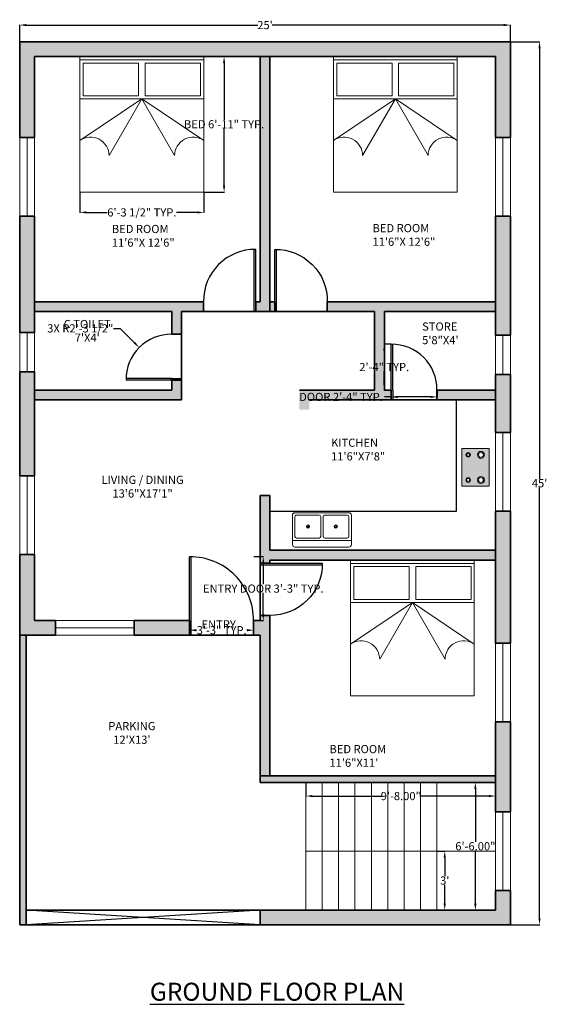
# Model space of a CAD drawing. Units: inches. Extents: x 107756 to 108945, y 133180 to 133782.
# Tile 3 of 3: x 108623 to 108945, y 133180 to 133782. Entities that reach past the tile are written whole.
import ezdxf

# ---------------------------------------------------------------- set-up
doc = ezdxf.new("R2010")
doc.units = ezdxf.units.IN
for name, color, linetype, lineweight in [('A-ANNO-DIMS', 2, 'Continuous', 13), ('A-ANNO-TEXT', 7, 'Continuous', 25), ('A-AREA-IDEN', 7, 'Continuous', 18), ('A-CASE', 8, 'Continuous', 25), ('A-DOOR', 3, 'Continuous', 25), ('A-EQPM', 8, 'Continuous', 18), ('A-FLOR-FIXT', 9, 'Continuous', 18), ('A-FLOR-STRS', 7, 'Continuous', 18), ('A-FURN', 8, 'Continuous', 18), ('A-GLAZ', 5, 'Continuous', 18), ('A-WALL', 7, 'Continuous', 35), ('A-WALL-PATT', 252, 'Continuous', 13)]:
    doc.layers.add(name, color=color, linetype=linetype, lineweight=lineweight)
doc.styles.get("Standard").update_dxf_attribs({"font": 'arial.ttf', "height": 5})
doc.styles.add('style1', font='arial.ttf', dxfattribs={"height": 11})
doc.dimstyles.get("Standard").update_dxf_attribs({"dimtxt": 5, "dimasz": 4, "dimexe": 0.18, "dimexo": 0.0625, "dimgap": 0.09, "dimtad": 0, "dimtih": 1, "dimtoh": 1, "dimzin": 0, "dimdsep": 46, "dimlunit": 3, "dimtxsty": 'Standard', "dimcen": 0.09, "dimclrd": 7, "dimclre": 256, "dimclrt": 256, "dimadec": 0, "dimazin": 0, "dimtfac": 1, "dimtofl": 0, "dimtmove": 0, "dimatfit": 3, "dimfxl": 1, "dimtolj": 1, "dimtzin": 0, "dimarcsym": 0})

# ---------------------------------------------------------------- blocks, each defined once
blk = doc.blocks.new('*D32')
at = {"layer": 'A-ANNO-DIMS', "color": 0, "lineweight": -2, "transparency": 16777216}
for p, q in [((108622.85, 133769.03), (108622.85, 133779.36)), ((108626.85, 133779.18), (108768.47, 133779.18)), ((108918.85, 133779.18), (108777.22, 133779.18)), ((108922.85, 133769.03), (108922.85, 133779.36))]:
    blk.add_line(p, q, dxfattribs=at)
at = {"layer": 'A-ANNO-DIMS', "color": 0, "transparency": 16777216}
for points in [[(108626.85, 133779.85), (108626.85, 133778.52), (108622.85, 133779.18)], [(108918.85, 133779.85), (108918.85, 133778.52), (108922.85, 133779.18)]]:
    blk.add_solid(points, dxfattribs=at)
at = {"layer": 'Defpoints', "color": 0, "transparency": 16777216}
for p in [(108922.85, 133779.18), (108622.85, 133768.97), (108922.85, 133768.97)]:
    blk.add_point(p, dxfattribs=at)
at = {"layer": 'A-ANNO-DIMS', "color": 0, "transparency": 16777216, "insert": (108772.85, 133779.18), "char_height": 5, "attachment_point": 5}
blk.add_mtext("\\A1;25'", dxfattribs=at)
blk = doc.blocks.new('*D33')
at = {"layer": 'A-ANNO-DIMS', "color": 0, "lineweight": -2, "transparency": 16777216}
for p, q in [((108922.91, 133768.97), (108940.88, 133768.97)), ((108940.7, 133764.97), (108940.7, 133501.6)), ((108940.7, 133232.97), (108940.7, 133496.34)), ((108922.91, 133228.97), (108940.88, 133228.97))]:
    blk.add_line(p, q, dxfattribs=at)
at = {"layer": 'A-ANNO-DIMS', "color": 0, "transparency": 16777216}
for points in [[(108940.04, 133764.97), (108941.37, 133764.97), (108940.7, 133768.97)], [(108940.04, 133232.97), (108941.37, 133232.97), (108940.7, 133228.97)]]:
    blk.add_solid(points, dxfattribs=at)
at = {"layer": 'Defpoints', "color": 0, "transparency": 16777216}
for p in [(108922.85, 133768.97), (108922.85, 133228.97), (108940.7, 133228.97)]:
    blk.add_point(p, dxfattribs=at)
at = {"layer": 'A-ANNO-DIMS', "color": 0, "transparency": 16777216, "insert": (108940.7, 133498.97), "char_height": 5, "attachment_point": 5}
blk.add_mtext("\\A1;45'", dxfattribs=at)
blk = doc.blocks.new('*D34')
at = {"layer": 'A-ANNO-DIMS', "color": 0, "lineweight": -2, "transparency": 16777216}
for p, q in [((108797.85, 133315.91), (108797.85, 133307.48)), ((108913.85, 133315.91), (108913.85, 133307.48)), ((108801.85, 133307.66), (108844.26, 133307.66)), ((108909.85, 133307.66), (108867.44, 133307.66))]:
    blk.add_line(p, q, dxfattribs=at)
at = {"layer": 'A-ANNO-DIMS', "color": 0, "transparency": 16777216}
for points in [[(108801.85, 133308.33), (108801.85, 133307), (108797.85, 133307.66)], [(108909.85, 133308.33), (108909.85, 133307), (108913.85, 133307.66)]]:
    blk.add_solid(points, dxfattribs=at)
at = {"layer": 'Defpoints', "color": 0, "transparency": 16777216}
for p in [(108797.85, 133315.97), (108913.85, 133315.97), (108797.85, 133307.66)]:
    blk.add_point(p, dxfattribs=at)
at = {"layer": 'A-ANNO-DIMS', "color": 0, "transparency": 16777216, "insert": (108855.85, 133307.66), "char_height": 5, "attachment_point": 5}
blk.add_mtext('\\A1;9\'-8.00"', dxfattribs=at)
blk = doc.blocks.new('*D35')
at = {"layer": 'A-ANNO-DIMS', "color": 0, "lineweight": -2, "transparency": 16777216}
for p, q in [((108913.78, 133315.97), (108901.27, 133315.97)), ((108901.45, 133311.97), (108901.45, 133279.61)), ((108901.45, 133241.97), (108901.45, 133274.33)), ((108913.78, 133237.97), (108901.27, 133237.97))]:
    blk.add_line(p, q, dxfattribs=at)
at = {"layer": 'A-ANNO-DIMS', "color": 0, "transparency": 16777216}
for points in [[(108900.78, 133311.97), (108902.12, 133311.97), (108901.45, 133315.97)], [(108900.78, 133241.97), (108902.12, 133241.97), (108901.45, 133237.97)]]:
    blk.add_solid(points, dxfattribs=at)
at = {"layer": 'Defpoints', "color": 0, "transparency": 16777216}
for p in [(108901.45, 133315.97), (108913.85, 133315.97), (108913.85, 133237.97)]:
    blk.add_point(p, dxfattribs=at)
at = {"layer": 'A-ANNO-DIMS', "color": 0, "transparency": 16777216, "insert": (108901.45, 133276.97), "char_height": 5, "attachment_point": 5}
blk.add_mtext('\\A1;6\'-6.00"', dxfattribs=at)
blk = doc.blocks.new('*D36')
at = {"layer": 'A-ANNO-DIMS', "color": 0, "lineweight": -2, "transparency": 16777216}
for p, q in [((108877.91, 133273.97), (108882.91, 133273.97)), ((108882.73, 133269.97), (108882.73, 133258.62)), ((108882.73, 133241.97), (108882.73, 133253.33)), ((108877.91, 133237.97), (108882.91, 133237.97))]:
    blk.add_line(p, q, dxfattribs=at)
at = {"layer": 'A-ANNO-DIMS', "color": 0, "transparency": 16777216}
for points in [[(108882.06, 133269.97), (108883.39, 133269.97), (108882.73, 133273.97)], [(108882.06, 133241.97), (108883.39, 133241.97), (108882.73, 133237.97)]]:
    blk.add_solid(points, dxfattribs=at)
at = {"layer": 'Defpoints', "color": 0, "transparency": 16777216}
for p in [(108877.85, 133273.97), (108882.73, 133273.97), (108877.85, 133237.97)]:
    blk.add_point(p, dxfattribs=at)
at = {"layer": 'A-ANNO-DIMS', "color": 0, "transparency": 16777216, "insert": (108882.73, 133255.97), "char_height": 5, "attachment_point": 5}
blk.add_mtext("\\A1;3'", dxfattribs=at)
blk = doc.blocks.new('NEW BED')
for p, q in [((-75.7, 82.92), (0, 82.92)), ((-75.7, 0), (-75.7, 82.92)), ((-75.7, 80.92), (0, 80.92)), ((-73.7, 78.92), (-39.85, 78.92)), ((-73.7, 58.92), (-73.7, 78.92)), ((-39.85, 58.92), (-39.85, 78.92)), ((-35.85, 78.92), (-2, 78.92)), ((-35.85, 58.92), (-35.85, 78.92)), ((-2, 78.92), (-2, 58.92)), ((0, 82.92), (0, 0)), ((-75.7, 56.92), (0, 56.92)), ((-37.85, 56.92), (-75.7, 31.45)), ((-73.7, 58.92), (-39.85, 58.92)), ((-37.85, 56.92), (-57.85, 22.27)), ((-37.85, 56.92), (0, 31.45)), ((-37.85, 56.92), (-17.84, 22.27)), ((-35.85, 58.92), (-2, 58.92)), ((0, 0), (-75.7, 0))]:
    blk.add_line(p, q)
for centre, start, end in [((-69.14, 22.27), 0, 125.54966), ((-6.56, 22.27), 54.45034, 180)]:
    blk.add_arc(centre, 11.28, start, end)
blk = doc.blocks.new('stov')
h = blk.add_hatch(color=256)
h.dxf.hatch_style = 1
h.set_gradient(color1=(255, 255, 255), color2=(147, 149, 152), name='CYLINDER')
h.paths.add_polyline_path([(0, 0), (16.67, 0), (16.67, 23.1), (0, 23.1)])
h.paths.add_polyline_path([(2.78, 19.21, -1), (7.12, 19.21, -1)], flags=16)
h.paths.add_polyline_path([(3.47, 19.21, -1), (6.43, 19.21, -1)], flags=0)
h.paths.add_polyline_path([(7.12, 3.89, -1), (2.78, 3.89, -1)], flags=16)
h.paths.add_polyline_path([(6.43, 3.89, -1), (3.47, 3.89, -1)], flags=0)
h.paths.add_polyline_path([(11.35, 19.27, -1), (14.15, 19.27, -1)], flags=16)
h.paths.add_polyline_path([(11.81, 19.27, -1), (13.68, 19.27, -1)], flags=0)
h.paths.add_polyline_path([(14.15, 3.83, -1), (11.35, 3.83, -1)], flags=16)
blk.add_lwpolyline([(16.67, 0), (0, 0), (0, 23.1), (16.67, 23.1)], close=True)
for centre, radius in [((4.95, 19.21), 2.17), ((4.95, 19.21), 2.17), ((4.95, 19.21), 1.48), ((12.75, 19.27), 1.4), ((12.75, 19.27), 0.936), ((4.95, 3.89), 2.17), ((4.95, 3.89), 2.17), ((4.95, 3.89), 1.48), ((12.75, 3.83), 1.4), ((12.75, 3.83), 0.936)]:
    blk.add_circle(centre, radius)
blk = doc.blocks.new('Sink-double - 36 in top')
for p, q in [((-18, -4), (18, -4)), ((-0.75, -18.5), (-0.75, -6.5)), ((0.75, -6.5), (0.75, -18.5))]:
    blk.add_line(p, q)
for points in [[(-16.5, 0), (16.5, 0)], [(-18, -19.5), (-18, -1.5)], [(-15.5, -5.5), (-1.75, -5.5)], [(1.75, -5.5), (15.5, -5.5)], [(18, -1.5), (18, -19.5)], [(-16.5, -18.5), (-16.5, -6.5)], [(16.5, -6.5), (16.5, -18.5)], [(16.5, -21), (-16.5, -21)], [(-1.75, -19.5), (-15.5, -19.5)], [(15.5, -19.5), (1.75, -19.5)]]:
    blk.add_lwpolyline(points)
for centre, radius in [((-8.5, -12.5), 1), ((-8.5, -12.5), 0.5), ((8.5, -12.5), 1), ((8.5, -12.5), 0.5)]:
    blk.add_circle(centre, radius)
for centre, radius, start, end in [((-16.5, -1.5), 1.5, 90, 180), ((16.5, -1.5), 1.5, 0, 90), ((-15.5, -6.5), 1, 90, 180), ((-1.75, -6.5), 1, 0, 90), ((1.75, -6.5), 1, 90, 180), ((15.5, -6.5), 1, 0, 90), ((-16.5, -19.5), 1.5, 180, 270), ((-15.5, -18.5), 1, 180, 270), ((-1.75, -18.5), 1, 270, 0), ((1.75, -18.5), 1, 180, 270), ((15.5, -18.5), 1, 270, 0), ((16.5, -19.5), 1.5, 270, 0)]:
    blk.add_arc(centre, radius, start, end)
blk = doc.blocks.new('DOOR-SWING-28IN')
for p, q in [((0, 28), (28, 28)), ((0, 27), (28, 27))]:
    blk.add_line(p, q)
blk.add_arc((0.5, 27.5), 27.5, 268.95837, 1.04163)
blk = doc.blocks.new('DOOR-SWING-32IN')
for p, q in [((0, 1), (32, 1)), ((0, 0), (32, 0))]:
    blk.add_line(p, q)
blk.add_arc((0.5, 0.5), 31.5, 359.09062, 90.90938)
blk = doc.blocks.new('DOOR-SWING-39IN')
for p, q in [((0, 0), (0, 39)), ((1, 0), (1, 39))]:
    blk.add_line(p, q)
blk.add_arc((0.5, 0.5), 38.5, 359.25594, 90.74406)
blk = doc.blocks.new('WIN-48IN')
blk.add_line((48, 4.5), (0, 4.5))
blk.add_lwpolyline([(0, 0), (48, 0), (48, 9), (0, 9)], close=True)
blk = doc.blocks.new('WIN-24IN')
blk.add_line((0, 4.5), (24, 4.5))
blk.add_lwpolyline([(0, 9), (24, 9), (24, 0), (0, 0)], close=True)
blk = doc.blocks.new('*D55')
at = {"layer": 'A-ANNO-DIMS', "lineweight": -2, "transparency": 16777216}
for p, q in [((108849.95, 133555.91), (108849.95, 133551.57)), ((108878.09, 133555.91), (108878.09, 133551.57))]:
    blk.add_line(p, q, dxfattribs=at)
at = {"layer": 'A-ANNO-DIMS', "color": 7, "lineweight": -2, "transparency": 16777216}
for p, q in [((108849.95, 133551.75), (108845.95, 133551.75)), ((108874.09, 133551.75), (108853.95, 133551.75))]:
    blk.add_line(p, q, dxfattribs=at)
at = {"layer": 'A-ANNO-DIMS', "color": 7, "transparency": 16777216}
for points in [[(108853.95, 133552.42), (108853.95, 133551.08), (108849.95, 133551.75)], [(108874.09, 133552.42), (108874.09, 133551.08), (108878.09, 133551.75)]]:
    blk.add_solid(points, dxfattribs=at)
at = {"layer": 'Defpoints', "color": 0, "transparency": 16777216}
for p in [(108849.95, 133555.97), (108878.09, 133555.97), (108849.95, 133551.75)]:
    blk.add_point(p, dxfattribs=at)
at = {"layer": 'A-ANNO-DIMS', "transparency": 16777216, "insert": (108819.3, 133551.75), "char_height": 5, "attachment_point": 5}
blk.add_mtext('\\A1;DOOR 2\'-4" TYP.', dxfattribs=at)
blk = doc.blocks.new('*D56')
at = {"layer": 'A-ANNO-DIMS', "lineweight": -2, "transparency": 16777216}
for p, q in [((108849.89, 133584.11), (108845.55, 133584.11)), ((108849.89, 133555.97), (108845.55, 133555.97))]:
    blk.add_line(p, q, dxfattribs=at)
at = {"layer": 'A-ANNO-DIMS', "color": 7, "lineweight": -2, "transparency": 16777216}
for p, q in [((108845.73, 133580.11), (108845.73, 133572.64)), ((108845.73, 133559.97), (108845.73, 133567.44))]:
    blk.add_line(p, q, dxfattribs=at)
at = {"layer": 'A-ANNO-DIMS', "color": 7, "transparency": 16777216}
for points in [[(108845.07, 133580.11), (108846.4, 133580.11), (108845.73, 133584.11)], [(108845.07, 133559.97), (108846.4, 133559.97), (108845.73, 133555.97)]]:
    blk.add_solid(points, dxfattribs=at)
at = {"layer": 'Defpoints', "color": 0, "transparency": 16777216}
for p in [(108845.73, 133584.11), (108849.95, 133584.11), (108849.95, 133555.97)]:
    blk.add_point(p, dxfattribs=at)
at = {"layer": 'A-ANNO-DIMS', "transparency": 16777216, "insert": (108845.73, 133570.04), "char_height": 5, "attachment_point": 5}
blk.add_mtext('\\A1;2\'-4" TYP.', dxfattribs=at)
blk = doc.blocks.new('*D57')
at = {"layer": 'A-ANNO-DIMS', "lineweight": -2, "transparency": 16777216}
for p, q in [((108765.96, 133454.11), (108771.95, 133454.11)), ((108765.96, 133414.97), (108771.95, 133414.97))]:
    blk.add_line(p, q, dxfattribs=at)
at = {"layer": 'A-ANNO-DIMS', "color": 7, "lineweight": -2, "transparency": 16777216}
for p, q in [((108771.77, 133450.11), (108771.77, 133437.22)), ((108771.77, 133418.97), (108771.77, 133431.86))]:
    blk.add_line(p, q, dxfattribs=at)
at = {"layer": 'A-ANNO-DIMS', "color": 7, "transparency": 16777216}
for points in [[(108771.1, 133450.11), (108772.43, 133450.11), (108771.77, 133454.11)], [(108771.1, 133418.97), (108772.43, 133418.97), (108771.77, 133414.97)]]:
    blk.add_solid(points, dxfattribs=at)
at = {"layer": 'Defpoints', "color": 0, "transparency": 16777216}
for p in [(108765.9, 133454.11), (108771.77, 133454.11), (108765.9, 133414.97)]:
    blk.add_point(p, dxfattribs=at)
at = {"layer": 'A-ANNO-DIMS', "transparency": 16777216, "insert": (108771.77, 133434.54), "char_height": 5, "attachment_point": 5}
blk.add_mtext('\\A1;ENTRY DOOR 3\'-3" TYP.', dxfattribs=at)
blk = doc.blocks.new('*D58')
at = {"layer": 'A-ANNO-DIMS', "lineweight": -2, "transparency": 16777216}
for p, q in [((108726.76, 133414.91), (108726.76, 133408.92)), ((108765.9, 133414.91), (108765.9, 133408.92))]:
    blk.add_line(p, q, dxfattribs=at)
at = {"layer": 'A-ANNO-DIMS', "color": 7, "lineweight": -2, "transparency": 16777216}
for p, q in [((108730.76, 133409.1), (108731, 133409.1)), ((108761.9, 133409.1), (108761.66, 133409.1))]:
    blk.add_line(p, q, dxfattribs=at)
at = {"layer": 'A-ANNO-DIMS', "color": 7, "transparency": 16777216}
for points in [[(108730.76, 133409.77), (108730.76, 133408.43), (108726.76, 133409.1)], [(108761.9, 133409.77), (108761.9, 133408.43), (108765.9, 133409.1)]]:
    blk.add_solid(points, dxfattribs=at)
at = {"layer": 'Defpoints', "color": 0, "transparency": 16777216}
for p in [(108726.76, 133414.97), (108765.9, 133414.97), (108765.9, 133409.1)]:
    blk.add_point(p, dxfattribs=at)
at = {"layer": 'A-ANNO-DIMS', "transparency": 16777216, "insert": (108746.33, 133409.1), "char_height": 5, "attachment_point": 5}
blk.add_mtext('\\A1;3\'-3" TYP.', dxfattribs=at)
blk = doc.blocks.new('*D59')
at = {"layer": 'A-ANNO-DIMS', "lineweight": -2, "transparency": 16777216}
for p, q in [((108735.45, 133759.97), (108748, 133759.97)), ((108735.45, 133677.05), (108748, 133677.05))]:
    blk.add_line(p, q, dxfattribs=at)
at = {"layer": 'A-ANNO-DIMS', "color": 7, "lineweight": -2, "transparency": 16777216}
for p, q in [((108747.82, 133755.97), (108747.82, 133721.15)), ((108747.82, 133681.05), (108747.82, 133715.87))]:
    blk.add_line(p, q, dxfattribs=at)
at = {"layer": 'A-ANNO-DIMS', "color": 7, "transparency": 16777216}
for points in [[(108747.15, 133755.97), (108748.49, 133755.97), (108747.82, 133759.97)], [(108747.15, 133681.05), (108748.49, 133681.05), (108747.82, 133677.05)]]:
    blk.add_solid(points, dxfattribs=at)
at = {"layer": 'Defpoints', "color": 0, "transparency": 16777216}
for p in [(108735.38, 133759.97), (108747.82, 133759.97), (108735.38, 133677.05)]:
    blk.add_point(p, dxfattribs=at)
at = {"layer": 'A-ANNO-DIMS', "transparency": 16777216, "insert": (108747.82, 133718.51), "char_height": 5, "attachment_point": 5}
blk.add_mtext('\\A1;BED 6\'-11" TYP.', dxfattribs=at)
blk = doc.blocks.new('*D60')
at = {"layer": 'A-ANNO-DIMS', "lineweight": -2, "transparency": 16777216}
for p, q in [((108659.68, 133676.99), (108659.68, 133664.43)), ((108735.38, 133676.99), (108735.38, 133664.43))]:
    blk.add_line(p, q, dxfattribs=at)
at = {"layer": 'A-ANNO-DIMS', "color": 7, "lineweight": -2, "transparency": 16777216}
for p, q in [((108663.68, 133664.61), (108676.37, 133664.61)), ((108731.38, 133664.61), (108718.7, 133664.61))]:
    blk.add_line(p, q, dxfattribs=at)
at = {"layer": 'A-ANNO-DIMS', "color": 7, "transparency": 16777216}
for points in [[(108663.68, 133665.28), (108663.68, 133663.94), (108659.68, 133664.61)], [(108731.38, 133665.28), (108731.38, 133663.94), (108735.38, 133664.61)]]:
    blk.add_solid(points, dxfattribs=at)
at = {"layer": 'Defpoints', "color": 0, "transparency": 16777216}
for p in [(108659.68, 133677.05), (108735.38, 133677.05), (108735.38, 133664.61)]:
    blk.add_point(p, dxfattribs=at)
at = {"layer": 'A-ANNO-DIMS', "transparency": 16777216, "insert": (108697.53, 133664.61), "char_height": 5, "attachment_point": 5}
blk.add_mtext('\\A1;6\'-3 1/2" TYP.', dxfattribs=at)
blk = doc.blocks.new('*D69')
at = {"layer": 'A-ANNO-DIMS', "color": 7, "lineweight": -2, "transparency": 16777216}
for p, q in [((108680.23, 133593.69), (108684.23, 133593.69)), ((108684.23, 133593.69), (108693.07, 133584.84))]:
    blk.add_line(p, q, dxfattribs=at)
at = {"layer": 'A-ANNO-DIMS', "lineweight": -2, "transparency": 16777216}
for p, q in [((108715.26, 133562.57), (108715.44, 133562.57)), ((108715.35, 133562.48), (108715.35, 133562.66))]:
    blk.add_line(p, q, dxfattribs=at)
at = {"layer": 'A-ANNO-DIMS', "color": 7, "transparency": 16777216}
blk.add_solid([(108693.54, 133585.32), (108692.6, 133584.37), (108695.9, 133582.02)], dxfattribs=at)
at = {"layer": 'Defpoints', "color": 0, "transparency": 16777216}
for p in [(108695.9, 133582.02), (108715.35, 133562.57)]:
    blk.add_point(p, dxfattribs=at)
at = {"layer": 'A-ANNO-DIMS', "transparency": 16777216, "insert": (108659.9, 133593.69), "char_height": 5, "attachment_point": 5}
blk.add_mtext('\\A1;3X R2\'-3 1/2"', dxfattribs=at)

msp = doc.modelspace()

# ---------------------------------------------------------------- hatches: boundary and pattern name
at = {"layer": 'A-WALL-PATT'}
h = msp.add_hatch(color=256, dxfattribs=at)
h.dxf.hatch_style = 1
h.paths.add_polyline_path([(108631.847, 133455.469), (108622.847, 133455.469), (108622.847, 133405.971), (108644.833, 133405.971), (108644.833, 133414.971), (108631.847, 133414.971)])
h.paths.add_polyline_path([(108726.761, 133414.971), (108692.833, 133414.971), (108692.833, 133405.971), (108726.761, 133405.971)])
h.paths.add_polyline_path([(108631.847, 133567.129), (108622.847, 133567.129), (108622.847, 133503.469), (108631.847, 133503.469)])
h.paths.add_polyline_path([(108721.847, 133562.068), (108715.847, 133562.068), (108715.847, 133555.971), (108631.847, 133555.971), (108631.847, 133549.971), (108721.847, 133549.971)])
h.paths.add_polyline_path([(108735.245, 133609.971), (108631.847, 133609.971), (108631.847, 133603.971), (108715.847, 133603.971), (108715.847, 133590.068), (108721.847, 133590.068), (108721.847, 133603.971), (108735.245, 133603.971)])
h.paths.add_polyline_path([(108631.847, 133662.372), (108622.847, 133662.372), (108622.847, 133591.129), (108631.847, 133591.129)])
h.paths.add_polyline_path([(108631.847, 133759.971), (108913.847, 133759.971), (108913.847, 133710.372), (108922.847, 133710.372), (108922.847, 133768.971), (108622.847, 133768.971), (108622.847, 133710.372), (108631.847, 133710.372)])
h.paths.add_polyline_path([(108775.847, 133759.971), (108769.847, 133759.971), (108769.847, 133609.971), (108767.245, 133609.971), (108767.245, 133603.971), (108775.847, 133603.971)])
h.paths.add_polyline_path([(108913.847, 133609.971), (108810.91, 133609.971), (108810.91, 133603.971), (108839.847, 133603.971), (108839.847, 133555.971), (108793.885, 133555.971), (108793.885, 133549.971), (108793.885, 133543.971), (108799.885, 133543.971), (108799.885, 133549.971), (108849.953, 133549.971), (108849.953, 133555.971), (108845.847, 133555.971), (108845.847, 133603.971), (108913.847, 133603.971)])
h.paths.add_polyline_path([(108778.91, 133609.971), (108775.847, 133609.971), (108775.847, 133603.971), (108778.91, 133603.971)])
h.paths.add_polyline_path([(108922.847, 133565.518), (108913.847, 133565.518), (108913.847, 133529.971), (108922.847, 133529.971)])
h.paths.add_polyline_path([(108913.847, 133555.971), (108877.953, 133555.971), (108877.953, 133549.971), (108913.847, 133549.971)], flags=17)
h.paths.add_polyline_path([(108922.847, 133662.372), (108913.847, 133662.372), (108913.847, 133589.518), (108922.847, 133589.518)])
h.paths.add_polyline_path([(108922.847, 133481.971), (108913.847, 133481.971), (108913.847, 133401.109), (108922.847, 133401.109)])
h.paths.add_polyline_path([(108913.847, 133457.971), (108775.847, 133457.971), (108775.847, 133491.569), (108769.847, 133491.569), (108769.847, 133450.154), (108775.847, 133450.154), (108775.847, 133451.971), (108913.847, 133451.971)])
h.paths.add_polyline_path([(108775.847, 133418.154), (108769.847, 133418.154), (108769.847, 133414.971), (108765.761, 133414.971), (108765.761, 133405.971), (108769.847, 133405.971), (108769.847, 133319.971), (108775.847, 133319.971)])
h.paths.add_polyline_path([(108922.847, 133353.109), (108913.847, 133353.109), (108913.847, 133315.971), (108913.847, 133297.971), (108922.847, 133297.971)])
h.paths.add_polyline_path([(108913.847, 133319.971), (108769.847, 133319.971), (108769.847, 133315.971), (108913.847, 133315.971)])
h.paths.add_polyline_path([(108922.847, 133249.971), (108913.847, 133249.971), (108913.847, 133237.971), (108769.847, 133237.971), (108769.847, 133228.971), (108922.847, 133228.971)])
h.paths.add_polyline_path([(108626.847, 133405.971), (108622.847, 133405.971), (108622.847, 133228.971), (108626.847, 133228.971)])

# ---------------------------------------------------------------- linework, layer by layer
at = {"layer": 'A-CASE'}
for p, q in [((108889.847, 133481.971), (108889.847, 133549.971)), ((108775.847, 133481.971), (108889.847, 133481.971))]:
    msp.add_line(p, q, dxfattribs=at)
at = {"layer": 'A-DOOR'}
for p, q in [((108766.245, 133603.971), (108766.245, 133609.971)), ((108779.91, 133603.971), (108779.91, 133609.971)), ((108715.847, 133563.068), (108721.847, 133563.068)), ((108850.953, 133555.971), (108850.953, 133549.971)), ((108769.847, 133449.154), (108775.847, 133449.154)), ((108727.761, 133405.971), (108727.761, 133414.971)), ((108769.847, 133228.971), (108626.847, 133237.971)), ((108769.847, 133237.971), (108626.847, 133228.971))]:
    msp.add_line(p, q, dxfattribs=at)
at = {"layer": 'A-FLOR-STRS'}
for p, q in [((108797.847, 133315.971), (108797.847, 133237.971)), ((108807.847, 133315.971), (108807.847, 133237.971)), ((108817.847, 133315.971), (108817.847, 133237.971)), ((108827.847, 133315.971), (108827.847, 133237.971)), ((108837.847, 133315.971), (108837.847, 133237.971)), ((108847.847, 133315.971), (108847.847, 133237.971)), ((108857.847, 133315.971), (108857.847, 133237.971)), ((108867.847, 133315.971), (108867.847, 133237.971)), ((108877.847, 133315.971), (108877.847, 133237.971)), ((108913.847, 133273.971), (108797.847, 133273.971))]:
    msp.add_line(p, q, dxfattribs=at)
at = {"layer": 'A-WALL'}
for p, q in [((108631.847, 133759.971), (108913.847, 133759.971)), ((108631.847, 133710.372), (108631.847, 133759.971)), ((108769.847, 133609.971), (108769.847, 133759.971)), ((108769.847, 133759.971), (108769.847, 133609.971)), ((108775.847, 133759.971), (108775.847, 133603.971)), ((108775.847, 133759.971), (108775.847, 133603.971)), ((108913.847, 133759.971), (108913.847, 133710.372)), ((108631.847, 133710.372), (108622.847, 133710.372)), ((108913.847, 133710.372), (108922.847, 133710.372)), ((108631.847, 133662.372), (108622.847, 133662.372)), ((108631.847, 133591.129), (108631.847, 133662.372)), ((108913.847, 133662.372), (108922.847, 133662.372)), ((108913.847, 133662.372), (108913.847, 133589.518)), ((108631.847, 133609.971), (108735.245, 133609.971)), ((108735.245, 133603.971), (108735.245, 133609.971)), ((108767.245, 133603.971), (108767.245, 133609.971)), ((108767.245, 133609.971), (108769.847, 133609.971)), ((108775.847, 133609.971), (108778.91, 133609.971)), ((108778.91, 133603.971), (108778.91, 133609.971)), ((108810.91, 133603.971), (108810.91, 133609.971)), ((108810.91, 133609.971), (108913.847, 133609.971)), ((108631.847, 133603.971), (108715.847, 133603.971)), ((108715.847, 133590.068), (108715.847, 133603.971)), ((108721.847, 133549.971), (108721.847, 133603.971)), ((108721.847, 133603.971), (108839.847, 133603.971)), ((108839.847, 133603.971), (108839.847, 133555.971)), ((108845.847, 133603.971), (108845.847, 133555.971)), ((108845.847, 133603.971), (108913.847, 133603.971)), ((108631.847, 133591.129), (108622.847, 133591.129)), ((108715.847, 133590.068), (108721.847, 133590.068)), ((108913.847, 133589.518), (108922.847, 133589.518)), ((108631.847, 133567.129), (108622.847, 133567.129)), ((108631.847, 133503.469), (108631.847, 133567.129)), ((108715.847, 133555.971), (108715.847, 133562.068)), ((108715.847, 133562.068), (108721.847, 133562.068)), ((108913.847, 133565.518), (108922.847, 133565.518)), ((108913.847, 133565.518), (108913.847, 133529.971)), ((108631.847, 133555.971), (108715.847, 133555.971)), ((108793.885, 133555.971), (108839.847, 133555.971)), ((108845.847, 133555.971), (108849.953, 133555.971)), ((108849.953, 133555.971), (108849.953, 133549.971)), ((108877.953, 133555.971), (108877.953, 133549.971)), ((108877.953, 133555.971), (108913.847, 133555.971)), ((108631.847, 133549.971), (108721.847, 133549.971)), ((108799.885, 133549.971), (108913.847, 133549.971)), ((108913.847, 133529.971), (108922.847, 133529.971)), ((108631.847, 133503.469), (108622.847, 133503.469)), ((108769.847, 133491.569), (108769.847, 133414.971)), ((108769.847, 133491.569), (108775.847, 133491.569)), ((108775.847, 133491.569), (108775.847, 133457.971)), ((108913.847, 133481.971), (108922.847, 133481.971)), ((108913.847, 133481.971), (108913.847, 133401.109)), ((108775.847, 133457.971), (108913.847, 133457.971)), ((108631.847, 133455.469), (108622.847, 133455.469)), ((108631.847, 133414.971), (108631.847, 133455.469)), ((108775.847, 133451.971), (108913.847, 133451.971)), ((108775.847, 133451.971), (108775.847, 133450.154)), ((108769.847, 133450.154), (108775.847, 133450.154)), ((108769.847, 133418.154), (108775.847, 133418.154)), ((108775.847, 133418.154), (108775.847, 133319.971)), ((108644.833, 133414.971), (108631.847, 133414.971)), ((108644.833, 133414.971), (108644.833, 133405.971)), ((108726.761, 133414.971), (108692.833, 133414.971)), ((108692.833, 133414.971), (108692.833, 133405.971)), ((108726.761, 133405.971), (108726.761, 133414.971)), ((108769.847, 133414.971), (108765.761, 133414.971)), ((108765.761, 133405.971), (108765.761, 133414.971)), ((108644.833, 133405.971), (108622.847, 133405.971)), ((108769.847, 133405.971), (108692.833, 133405.971)), ((108769.847, 133405.971), (108769.847, 133315.971)), ((108913.847, 133401.109), (108922.847, 133401.109)), ((108913.847, 133353.109), (108922.847, 133353.109)), ((108913.847, 133353.109), (108913.847, 133315.971)), ((108769.847, 133319.971), (108913.847, 133319.971)), ((108769.847, 133315.971), (108913.847, 133315.971)), ((108913.847, 133315.971), (108913.847, 133297.971)), ((108913.847, 133297.971), (108922.847, 133297.971)), ((108913.847, 133249.971), (108922.847, 133249.971)), ((108913.847, 133249.971), (108913.847, 133237.971)), ((108913.847, 133237.971), (108626.847, 133237.971)), ((108769.847, 133237.971), (108769.847, 133228.971))]:
    msp.add_line(p, q, dxfattribs=at)
for points in [[(108622.847, 133768.971), (108922.847, 133768.971), (108922.847, 133710.372)], [(108622.847, 133710.372), (108622.847, 133768.971)], [(108622.847, 133591.129), (108622.847, 133662.372)], [(108922.847, 133662.372), (108922.847, 133589.518)], [(108622.847, 133503.469), (108622.847, 133567.129)], [(108922.847, 133565.518), (108922.847, 133529.971)], [(108922.847, 133481.971), (108922.847, 133401.109)], [(108622.847, 133405.971), (108622.847, 133455.469)], [(108622.847, 133228.971), (108622.847, 133405.971)], [(108626.847, 133228.971), (108626.847, 133405.971)], [(108922.847, 133353.109), (108922.847, 133297.971)], [(108922.847, 133249.971), (108922.847, 133228.971), (108626.847, 133228.971)], [(108626.847, 133228.971), (108622.847, 133228.971)]]:
    msp.add_lwpolyline(points, dxfattribs=at)

# ---------------------------------------------------------------- block references
at = {"layer": 'A-DOOR'}
for name, p, rotation in [('DOOR-SWING-32IN', (108767.245, 133609.971), 90.00000000002534), ('DOOR-SWING-28IN', (108715.847, 133590.068), 180), ('DOOR-SWING-28IN', (108877.953, 133555.971), 90.00000000002858)]:
    msp.add_blockref(name, p, dxfattribs=dict(at, rotation=rotation))
at = {"layer": 'A-DOOR', "extrusion": (0, 0, -1), "zscale": -1}
for p, rotation in [((-108778.91, 133609.971), 89.99999999998802), ((-108775.847, 133450.154), 180)]:
    msp.add_blockref('DOOR-SWING-32IN', p, dxfattribs=dict(at, rotation=rotation))
at = {"layer": 'A-DOOR'}
msp.add_blockref('DOOR-SWING-39IN', (108726.761, 133414.971), dxfattribs=at)
at = {"layer": 'A-EQPM', "rotation": 180}
msp.add_blockref('stov', (108909.815, 133520.181), dxfattribs=at)
at = {"layer": 'A-FLOR-FIXT', "rotation": 180}
msp.add_blockref('Sink-double - 36 in top', (108807.629, 133459.938), dxfattribs=at)
at = {"layer": 'A-FURN'}
for p in [(108735.383, 133677.049), (108890.369, 133677.049), (108900.801, 133369.049)]:
    msp.add_blockref('NEW BED', p, dxfattribs=at)
at = {"layer": 'A-GLAZ'}
for p, rotation in [((108622.847, 133710.372), 269.9999999999652), ((108913.847, 133710.372), 269.9999999999652), ((108913.847, 133529.971), 269.9999999999761), ((108622.847, 133503.469), 269.9999999999761), ((108913.847, 133401.109), 269.9999999999761), ((108913.847, 133297.971), 269.9999999999761)]:
    msp.add_blockref('WIN-48IN', p, dxfattribs=dict(at, rotation=rotation))
at = {"layer": 'A-GLAZ', "extrusion": (0, 0, -1), "zscale": -1, "rotation": 269.9999999999667}
for p in [(-108631.847, 133591.129), (-108922.847, 133589.518)]:
    msp.add_blockref('WIN-24IN', p, dxfattribs=at)
at = {"layer": 'A-GLAZ'}
msp.add_blockref('WIN-48IN', (108644.833, 133405.971), dxfattribs=at)

# ---------------------------------------------------------------- texts
at = {"layer": 'A-ANNO-TEXT', "insert": (108702.432, 133193.501), "char_height": 11, "attachment_point": 1, "style": 'style1'}
msp.add_mtext_dynamic_manual_height_columns('{\\fArial|b1|i0|c0|p34;\\LGROUND FLOOR PLAN}', width=176.25425, gutter_width=55, heights=[0], dxfattribs=at)
at = {"layer": 'A-AREA-IDEN', "char_height": 5, "attachment_point": 1}
for s, width, insert in [('BED ROOM\\P11\'6"X 12\'6"', 75.0129, (108679.174, 133656.975)), ('BED ROOM\\P11\'6"X 12\'6"', 75.0129, (108838.563, 133657.499)), ("\\pxqc;C TOILET\\P7'X4'", 45.00921, (108641.648, 133598.833)), ('STORE\\P5\'8"X4\'', 26.11625, (108868.896, 133597.323)), ('KITCHEN\\P11\'6"X7\'8"', 32.24688, (108813.22, 133526.24)), ('\\pxqc;LIVING / DINING\\P13\'6"X17\'1"', 78.97199, (108658.495, 133503.544)), ('ENTRY', 28.74375, (108733.993, 133415.137)), ("\\pxqc;PARKING \\P12'X13'", 51.98988, (108665.448, 133352.946)), ('BED ROOM\\P11\'6"X11\'', 63.50663, (108812.24, 133338.885))]:
    msp.add_mtext_dynamic_manual_height_columns(s, width=width, gutter_width=25, heights=[0], dxfattribs=dict(at, insert=insert))

# ---------------------------------------------------------------- dimensions: what is measured, and where the dimension line sits
at = {"layer": 'A-ANNO-DIMS'}
for base, p1, p2, picture, middle in [((108922.847, 133779.184), (108622.847, 133768.971), (108922.847, 133768.971), '*D32', (108772.847, 133779.184)), ((108797.847, 133307.665), (108913.847, 133315.971), (108797.847, 133315.971), '*D34', (108855.847, 133307.665))]:
    dim = msp.add_linear_dim(base=base, p1=p1, p2=p2, dimstyle='Standard', override={"dimclrd": 0, "dimclre": 0, "dimclrt": 0}, dxfattribs=at)
    dim.commit()
    dim.dimension.update_dxf_attribs({"geometry": picture, "text_midpoint": middle})
dim = msp.add_linear_dim(base=(108940.702, 133228.971), p1=(108922.847, 133768.971), p2=(108922.847, 133228.971), angle=90, dimstyle='Standard', override={"dimclrd": 0, "dimclre": 0, "dimclrt": 0}, dxfattribs=at)
dim.commit()
dim.dimension.update_dxf_attribs({"geometry": '*D33', "text_midpoint": (108940.702, 133498.971), "dimtype": 160})
for base, p1, p2, angle, text, picture, middle in [((108747.822, 133759.971), (108735.383, 133677.049), (108735.383, 133759.971), 90, 'BED <> TYP.', '*D59', (108747.822, 133718.51)), ((108845.732, 133584.106), (108849.953, 133555.971), (108849.953, 133584.106), 90, '<> TYP.', '*D56', (108845.732, 133570.038)), ((108849.953, 133551.75), (108878.088, 133555.971), (108849.953, 133555.971), 180, 'DOOR <> TYP.', '*D55', (108819.301, 133551.75)), ((108771.766, 133454.105), (108765.895, 133414.971), (108765.895, 133454.105), 90, 'ENTRY DOOR <> TYP.', '*D57', (108771.766, 133434.538))]:
    dim = msp.add_linear_dim(base=base, p1=p1, p2=p2, angle=angle, text=text, dimstyle='Standard', override={"dimdec": 1, "dimlfac": 1, "dimrnd": 0, "dimzin": 1, "dimdsep": 46, "dimlunit": 4, "dimfrac": 2}, dxfattribs=at)
    dim.commit()
    dim.dimension.update_dxf_attribs({"geometry": picture, "text_midpoint": middle})
for base, p1, p2, picture, middle in [((108735.383, 133664.611), (108659.684, 133677.049), (108735.383, 133677.049), '*D60', (108697.534, 133664.611)), ((108765.895, 133409.1), (108726.761, 133414.971), (108765.895, 133414.971), '*D58', (108746.328, 133409.1))]:
    dim = msp.add_linear_dim(base=base, p1=p1, p2=p2, text='<> TYP.', dimstyle='Standard', override={"dimdec": 1, "dimlfac": 1, "dimrnd": 0, "dimzin": 1, "dimdsep": 46, "dimlunit": 4, "dimfrac": 2}, dxfattribs=at)
    dim.commit()
    dim.dimension.update_dxf_attribs({"geometry": picture, "text_midpoint": middle})
dim = msp.add_radius_dim(center=(108715.347, 133562.568), mpoint=(108695.898, 133582.016), text='3X <>', dimstyle='Standard', override={"dimdec": 1, "dimlfac": 1, "dimrnd": 0, "dimzin": 1, "dimdsep": 46, "dimlunit": 4, "dimfrac": 2}, dxfattribs=at)
dim.commit()
dim.dimension.update_dxf_attribs({"geometry": '*D69', "text_midpoint": (108659.905, 133593.685), "dimtype": 164})
for base, p1, p2, picture, middle in [((108901.45, 133315.971), (108913.847, 133237.971), (108913.847, 133315.971), '*D35', (108901.45, 133276.971)), ((108882.727, 133273.971), (108877.847, 133237.971), (108877.847, 133273.971), '*D36', (108882.727, 133255.971))]:
    dim = msp.add_linear_dim(base=base, p1=p1, p2=p2, angle=90, dimstyle='Standard', override={"dimclrd": 0, "dimclre": 0, "dimclrt": 0}, dxfattribs=at)
    dim.commit()
    dim.dimension.update_dxf_attribs({"geometry": picture, "text_midpoint": middle})

doc.saveas('drawing.dxf')
